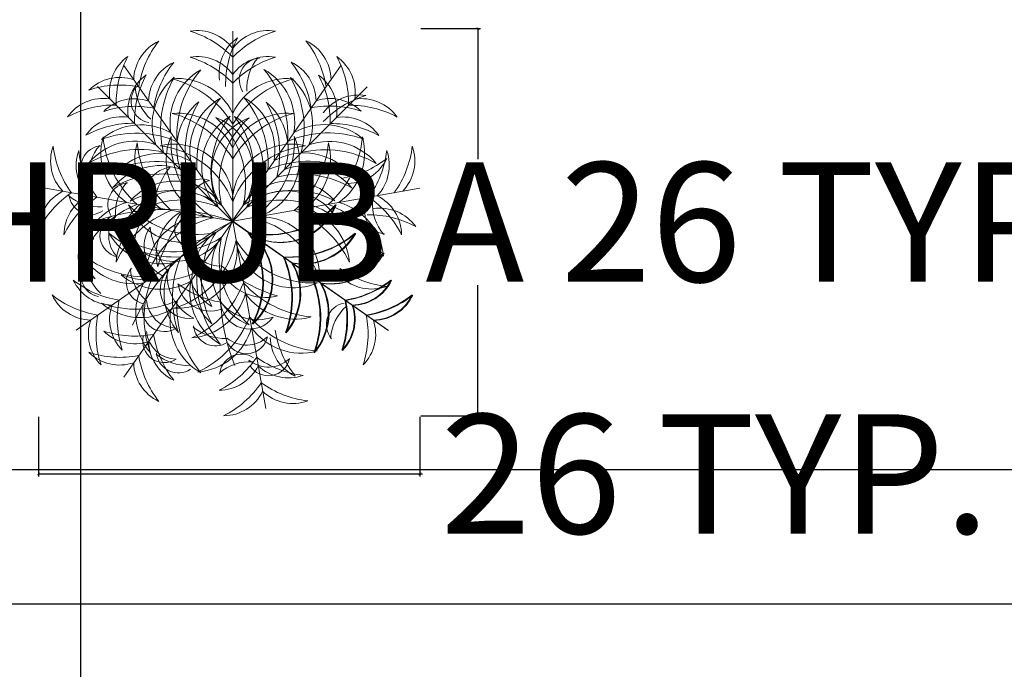
# Model space of a CAD drawing. Units: inches. Extents: x -48 to 50072, y 0 to 21068.
# Tile 5 of 75: x 212 to 278, y 210 to 253. Entities that reach past the tile are written whole.
import ezdxf

# ---------------------------------------------------------------- set-up
doc = ezdxf.new("R2010")
doc.units = ezdxf.units.IN
doc.header["$MEASUREMENT"] = 0
for name, color, linetype, lineweight in [('A-ANNO-DIMS', 2, 'Continuous', 18), ('C-PROP', 7, 'Continuous', 25), ('L-PLNT', 94, 'Continuous', 13)]:
    doc.layers.add(name, color=color, linetype=linetype, lineweight=lineweight)
doc.styles.get("Standard").update_dxf_attribs({"font": 'arial.ttf'})
doc.dimstyles.get("Standard").update_dxf_attribs({"dimtxt": 8, "dimasz": 0.18, "dimexe": 0.18, "dimexo": 0.0625, "dimgap": 0.09, "dimtad": 0, "dimtih": 1, "dimtoh": 1, "dimdec": 1, "dimzin": 0, "dimdsep": 46, "dimlunit": 4, "dimtxsty": 'Standard', "dimblk": 'ARCHTICK', "dimcen": 0.09, "dimadec": 0, "dimazin": 0, "dimtfac": 1, "dimtdec": 1, "dimtofl": 0, "dimtmove": 0, "dimatfit": 3, "dimldrblk": 'ARCHTICK', "dimfxl": 1, "dimtolj": 1, "dimtzin": 0, "dimarcsym": 0})

# ---------------------------------------------------------------- blocks, each defined once
blk = doc.blocks.new('A$C5D061C3B')
for p, q in [((3.377, 6.679), (3.377, 3.377)), ((1.483, 6.082), (3.377, 3.377)), ((5.259, 6.086), (3.365, 3.381)), ((1.03, 5.716), (3.365, 3.381)), ((5.712, 5.712), (3.377, 3.377)), ((0.125, 3.951), (3.377, 3.377)), ((6.629, 3.951), (3.377, 3.377)), ((0.66, 1.487), (3.365, 3.381)), ((1.483, 0.672), (3.377, 3.377)), ((6.07, 1.487), (3.365, 3.381)), ((3.951, 0.125), (3.377, 3.377)), ((6.082, 1.483), (3.377, 3.377))]:
    blk.add_line(p, q)
for centre, radius, start, end in [((2.763, 5.924), 0.762, 36.29, 99.6243), ((2.145, 5.032), 1.715, 44.0763, 73.3794), ((3.991, 5.924), 0.762, 80.3757, 143.71), ((4.61, 5.032), 1.715, 106.6206, 135.9237), ((2.419, 5.816), 0.762, 115.3757, 178.71), ((3.438, 5.44), 1.715, 141.6206, 170.9237), ((3.901, 5.939), 0.762, 125.3757, 188.71), ((4.969, 5.745), 1.715, 151.6206, 180.9237), ((3.305, 5.444), 1.715, 9.0763, 38.3794), ((4.323, 5.82), 0.762, 1.29, 64.6243), ((1.998, 5.617), 0.762, 125.3757, 188.71), ((3.066, 5.423), 1.715, 151.6206, 180.9237), ((2.763, 5.474), 0.762, 36.29, 99.6243), ((2.145, 4.581), 1.715, 44.0763, 73.3794), ((3.991, 5.474), 0.762, 80.3757, 143.71), ((4.61, 4.581), 1.715, 106.6206, 135.9237), ((3.871, 5.832), 0.38, 94.742, 213.7475), ((4.447, 5.681), 0.826, 139.618, 183.2106), ((4.744, 5.613), 0.762, 351.29, 54.6243), ((3.676, 5.419), 1.715, 359.0763, 28.3794), ((2.678, 5.447), 0.762, 115.3757, 178.71), ((3.696, 5.07), 1.715, 141.6206, 170.9237), ((3.344, 5.089), 1.056, 119.6063, 189.7511), ((4.177, 4.869), 1.77, 139.9634, 183.6288), ((3.398, 5.094), 1.056, 350.2489, 60.3937), ((2.565, 4.873), 1.77, 356.3712, 40.0366), ((4.064, 5.451), 0.762, 1.29, 64.6243), ((3.046, 5.075), 1.715, 9.0763, 38.3794), ((1.413, 5.111), 0.762, 71.29, 134.6243), ((2.317, 5.298), 0.762, 125.3757, 188.71), ((3.385, 5.104), 1.715, 151.6206, 180.9237), ((3.035, 5.062), 1.056, 129.6063, 199.7511), ((3.894, 4.989), 1.77, 149.9634, 193.6288), ((2.422, 4.799), 1.056, 25.2489, 95.3937), ((1.866, 4.14), 1.77, 31.3712, 75.0366), ((4.332, 4.799), 1.056, 84.6063, 154.7511), ((4.888, 4.14), 1.77, 104.9634, 148.6288), ((2.848, 4.985), 1.77, 346.3712, 30.0366), ((3.707, 5.058), 1.056, 340.2489, 50.3937), ((3.357, 5.1), 1.715, 359.0763, 28.3794), ((4.425, 5.294), 0.762, 351.29, 54.6243), ((1.419, 4.026), 1.715, 79.0763, 108.3794), ((1.991, 5.462), 0.38, 139.742, 258.7475), ((2.505, 5.763), 0.826, 184.618, 228.2106), ((1.13, 4.748), 0.762, 81.29, 144.6243), ((1.671, 4.742), 0.762, 71.29, 134.6243), ((3.688, 4.597), 1.056, 119.6063, 189.7511), ((4.522, 4.377), 1.77, 139.9634, 183.6288), ((2.221, 4.381), 1.77, 356.3712, 40.0366), ((3.054, 4.602), 1.056, 350.2489, 60.3937), ((5.071, 4.746), 0.762, 45.3757, 108.71), ((5.564, 4.807), 0.762, 80.3757, 143.71), ((6.182, 3.914), 1.715, 106.6206, 135.9237), ((5.613, 4.744), 0.762, 35.3757, 98.71), ((1.324, 3.68), 1.715, 89.0763, 118.3794), ((1.677, 3.657), 1.715, 79.0763, 108.3794), ((3.46, 4.637), 1.056, 129.6063, 199.7511), ((4.319, 4.565), 1.77, 149.9634, 193.6288), ((3.283, 4.633), 1.056, 340.2489, 50.3937), ((2.424, 4.56), 1.77, 346.3712, 30.0366), ((5.065, 3.661), 1.715, 71.6206, 100.9237), ((5.419, 3.676), 1.715, 61.6206, 90.9237), ((1.448, 4.43), 0.762, 81.29, 144.6243), ((2.422, 4.198), 1.056, 25.2489, 95.3937), ((1.866, 3.54), 1.77, 31.3712, 75.0366), ((3.868, 4.321), 1.029, 121.3654, 221.5741), ((4.556, 4.237), 1.557, 141.8122, 203.3335), ((4.035, 4.215), 1.029, 111.3654, 211.5741), ((2.707, 4.219), 1.029, 328.4259, 68.6346), ((2.044, 4.017), 1.557, 346.6665, 48.1878), ((4.698, 4.013), 1.557, 131.8122, 193.3335), ((4.332, 4.198), 1.056, 84.6063, 154.7511), ((4.888, 3.54), 1.77, 104.9634, 148.6288), ((2.187, 4.233), 1.557, 336.6665, 38.1878), ((2.875, 4.316), 1.029, 318.4259, 58.6346), ((5.294, 4.425), 0.762, 35.3757, 98.71), ((1.642, 3.362), 1.715, 89.0763, 118.3794), ((1.78, 3.994), 1.056, 60.2489, 130.3937), ((4.963, 3.998), 1.056, 49.6063, 119.7511), ((5.1, 3.357), 1.715, 61.6206, 90.9237), ((2.143, 4.564), 1.056, 164.6063, 234.7511), ((1.702, 3.136), 1.77, 66.3712, 110.0366), ((2.888, 4.998), 1.77, 184.9634, 228.6288), ((3.25, 4.435), 1.029, 156.3654, 256.5741), ((3.862, 4.761), 1.557, 176.8122, 238.3335), ((2.893, 4.761), 1.557, 301.6665, 3.1878), ((3.504, 4.435), 1.029, 283.4259, 23.6346), ((5.04, 3.14), 1.77, 69.9634, 113.6288), ((3.866, 4.998), 1.77, 311.3712, 355.0366), ((4.611, 4.564), 1.056, 305.2489, 15.3937), ((0.975, 4.424), 0.762, 160.3757, 223.71), ((1.962, 4.878), 1.715, 186.6206, 215.9237), ((1.12, 4.31), 0.38, 94.742, 213.7475), ((1.696, 4.159), 0.826, 139.618, 183.2106), ((1.685, 3.712), 1.056, 70.2489, 140.3937), ((1.757, 2.853), 1.77, 76.3712, 120.0366), ((2.734, 4.46), 1.056, 164.6063, 234.7511), ((3.48, 4.893), 1.77, 184.9634, 228.6288), ((2.358, 3.686), 1.029, 3.4259, 103.6346), ((1.93, 3.14), 1.557, 21.6665, 83.1878), ((4.397, 3.686), 1.029, 76.3654, 176.5741), ((4.824, 3.14), 1.557, 96.8122, 158.3335), ((3.275, 4.893), 1.77, 311.3712, 355.0366), ((4.02, 4.46), 1.056, 305.2489, 15.3937), ((5.058, 3.707), 1.056, 39.6063, 109.7511), ((4.793, 4.878), 1.715, 324.0763, 353.3794), ((5.779, 4.424), 0.762, 316.29, 19.6243), ((1.419, 4.346), 0.762, 160.3757, 223.71), ((2.405, 4.8), 1.715, 186.6206, 215.9237), ((2.124, 3.502), 1.056, 60.2489, 130.3937), ((4.618, 3.506), 1.056, 49.6063, 119.7511), ((4.985, 2.848), 1.77, 59.9634, 103.6288), ((4.988, 5.812), 1.715, 279.0763, 308.3794), ((5.365, 4.794), 0.762, 271.29, 334.6243), ((4.349, 4.8), 1.715, 324.0763, 353.3794), ((5.335, 4.346), 0.762, 316.29, 19.6243), ((2.109, 3.287), 1.056, 70.2489, 140.3937), ((2.046, 2.644), 1.77, 66.3712, 110.0366), ((2.387, 3.752), 0.574, 99.9865, 199.4034), ((3.599, 3.314), 1.651, 142.5759, 170.8942), ((4.696, 2.648), 1.77, 69.9634, 113.6288), ((4.633, 3.283), 1.056, 39.6063, 109.7511), ((2.182, 2.428), 1.77, 76.3712, 120.0366), ((2.84, 3.739), 0.372, 69.2257, 210.1279), ((4.56, 2.424), 1.77, 59.9634, 103.6288), ((1.588, 3.666), 0.38, 94.742, 213.7475), ((2.165, 3.515), 0.826, 139.618, 183.2106), ((2.365, 3.045), 1.029, 38.4259, 138.6346), ((3.109, 3.59), 0.515, 105.4398, 183.6694), ((4.377, 3.05), 1.029, 41.3654, 141.5741), ((0.762, 3.214), 0.762, 116.29, 179.6243), ((1.534, 2.451), 1.715, 124.0763, 153.3794), ((1.206, 3.136), 0.762, 116.29, 179.6243), ((1.977, 2.373), 1.715, 124.0763, 153.3794), ((1.062, 4.452), 0.826, 229.618, 273.2106), ((0.91, 3.875), 0.38, 184.742, 303.7475), ((2.426, 2.879), 1.029, 48.4259, 148.6346), ((2.328, 2.353), 1.557, 56.6665, 118.1878), ((4.414, 2.358), 1.557, 61.8122, 123.3335), ((4.316, 2.875), 1.029, 31.3654, 131.5741), ((4.777, 2.373), 1.715, 26.6206, 55.9237), ((5.549, 3.136), 0.762, 0.3757, 63.71), ((1.811, 2.684), 1.056, 105.2489, 175.3937), ((2.363, 2.022), 1.77, 111.3712, 155.0366), ((2.403, 2.58), 1.056, 105.2489, 175.3937), ((2.51, 2.191), 1.557, 66.6665, 128.1878), ((2.729, 4.702), 1.557, 221.8122, 283.3335), ((2.527, 4.039), 1.029, 201.3654, 301.5741), ((2.741, 3.253), 0.372, 114.2257, 255.1279), ((3.037, 3.338), 0.515, 150.4398, 228.6694), ((4.233, 2.187), 1.557, 51.8122, 113.3335), ((4.001, 4.702), 1.557, 256.6665, 318.1878), ((4.013, 4.698), 1.557, 256.6665, 318.1878), ((4.203, 4.039), 1.029, 238.4259, 338.6346), ((4.215, 4.035), 1.029, 238.4259, 338.6346), ((4.352, 2.58), 1.056, 4.6063, 74.7511), ((4.391, 2.022), 1.77, 24.9634, 68.6288), ((4.943, 2.684), 1.056, 4.6063, 74.7511), ((6.053, 3.533), 0.38, 146.2525, 265.258), ((6.629, 3.684), 0.826, 176.7894, 220.382), ((5.935, 2.842), 0.762, 35.3757, 98.71), ((2.185, 0.015), 3.567, 70.4772, 111.6585), ((1.447, 3.129), 0.376, 122.0577, 257.8533), ((1.751, 3.126), 0.529, 140.1845, 223.654), ((2.955, 1.917), 1.77, 111.3712, 155.0366), ((2.007, 3.071), 0.506, 93.8744, 233.9763), ((2.489, 2.932), 0.825, 128.7536, 199.097), ((2.896, 2.427), 1.029, 83.4259, 183.6346), ((3.359, 1.911), 1.557, 101.6665, 163.1878), ((2.903, 2.8), 0.855, 116.4477, 194.3672), ((4.744, 1.779), 2.789, 140.4007, 163.139), ((3.395, 1.911), 1.557, 16.8122, 78.3335), ((3.858, 2.427), 1.029, 356.3654, 96.5741), ((3.799, 1.917), 1.77, 24.9634, 68.6288), ((5.741, 1.774), 1.715, 61.6206, 90.9237), ((4.912, 0.157), 3.567, 115.4772, 156.6585), ((2.412, 2.943), 0.574, 144.9865, 244.4034), ((3.578, 3.49), 1.651, 187.5759, 215.8942), ((6.727, 2.189), 3.567, 160.4772, 201.6585), ((1.37, 2.745), 0.529, 140.1845, 223.654), ((2.145, 3.693), 1.056, 209.6063, 279.7511), ((2.365, 4.526), 1.77, 229.9634, 273.6288), ((2.328, 4.401), 1.557, 241.8122, 303.3335), ((3.697, 2.369), 1.029, 128.4259, 228.6346), ((4.389, 2.332), 1.557, 146.6665, 208.1878), ((4.698, 2.741), 1.557, 166.6665, 228.1878), ((2.341, 2.332), 1.557, 331.8122, 33.3335), ((2.353, 2.328), 1.557, 331.8122, 33.3335), ((3.033, 2.369), 1.029, 311.3654, 51.5741), ((3.045, 2.365), 1.029, 311.3654, 51.5741), ((4.365, 4.526), 1.77, 266.3712, 310.0366), ((4.377, 4.522), 1.77, 266.3712, 310.0366), ((4.585, 3.693), 1.056, 260.2489, 330.3937), ((4.597, 3.688), 1.056, 260.2489, 330.3937), ((1.067, 2.749), 0.376, 122.0577, 257.8533), ((2.365, 3.709), 1.029, 221.3654, 321.5741), ((1.911, 3.359), 1.557, 286.8122, 348.3335), ((2.427, 2.896), 1.029, 266.3654, 6.5741), ((3.003, 2.844), 0.372, 159.2257, 300.1279), ((3.152, 3.113), 0.515, 195.4398, 273.6694), ((5.474, 3.214), 2.789, 185.4007, 208.139), ((4.035, 2.539), 1.029, 148.4259, 248.6346), ((4.435, 3.25), 1.029, 193.4259, 293.6346), ((4.761, 3.862), 1.557, 211.6665, 273.1878), ((1.873, 4.181), 1.77, 229.9634, 273.6288), ((1.653, 3.348), 1.056, 209.6063, 279.7511), ((4.099, 2.051), 1.77, 156.3712, 200.0366), ((3.45, 2.634), 0.855, 161.4477, 239.3672), ((2.632, 2.051), 1.77, 339.9634, 23.6288), ((2.644, 2.046), 1.77, 339.9634, 23.6288), ((4.857, 4.181), 1.77, 266.3712, 310.0366), ((4.869, 4.177), 1.77, 266.3712, 310.0366), ((5.077, 3.348), 1.056, 260.2489, 330.3937), ((5.089, 3.344), 1.056, 260.2489, 330.3937), ((1.122, 2.441), 0.38, 139.742, 258.7475), ((1.636, 2.741), 0.826, 184.618, 228.2106), ((3.24, 2.128), 1.056, 150.2489, 220.3937), ((4.963, 4.749), 2.789, 230.4007, 253.139), ((3.49, 2.128), 1.056, 319.6063, 29.7511), ((3.502, 2.124), 1.056, 319.6063, 29.7511), ((2.046, 4.111), 1.77, 249.9634, 293.6288), ((2.124, 3.252), 1.056, 229.6063, 299.7511), ((1.908, 2.317), 0.38, 139.742, 258.7475), ((2.422, 2.617), 0.826, 184.618, 228.2106), ((3.607, 1.706), 1.77, 156.3712, 200.0366), ((2.624, 2.192), 0.506, 138.8744, 278.9763), ((3.064, 2.435), 0.825, 173.7536, 244.097), ((4.522, 2.378), 1.77, 176.3712, 220.0366), ((3.942, 2.908), 0.855, 206.4477, 284.3672), ((3.124, 1.706), 1.77, 339.9634, 23.6288), ((3.136, 1.702), 1.77, 339.9634, 23.6288), ((6.244, 3.948), 1.715, 234.0763, 263.3794), ((5.79, 2.962), 0.762, 226.29, 289.6243), ((1.672, 3.7), 1.715, 231.6206, 260.9237), ((1.295, 2.682), 0.762, 205.3757, 268.71), ((2.748, 1.784), 1.056, 150.2489, 220.3937), ((3.428, 3.603), 1.651, 232.5759, 260.8942), ((2.99, 2.391), 0.574, 189.9865, 289.4034), ((3.688, 2.157), 1.056, 170.2489, 240.3937), ((1.917, 2.955), 1.77, 294.9634, 338.6288), ((4.893, 3.48), 1.77, 221.3712, 265.0366), ((3.982, 1.784), 1.056, 319.6063, 29.7511), ((3.994, 1.78), 1.056, 319.6063, 29.7511), ((5.058, 3.7), 1.715, 279.0763, 308.3794), ((5.07, 3.696), 1.715, 279.0763, 308.3794), ((5.435, 2.682), 0.762, 271.29, 334.6243), ((5.447, 2.678), 0.762, 271.29, 334.6243), ((0.926, 2.424), 0.762, 205.3757, 268.71), ((1.303, 3.442), 1.715, 231.6206, 260.9237), ((2.58, 2.403), 1.056, 274.6063, 344.7511), ((4.46, 2.734), 1.056, 215.2489, 285.3937), ((5.427, 3.442), 1.715, 279.0763, 308.3794), ((5.44, 3.438), 1.715, 279.0763, 308.3794), ((5.804, 2.424), 0.762, 271.29, 334.6243), ((5.816, 2.419), 0.762, 271.29, 334.6243), ((1.702, 3.619), 1.77, 249.9634, 293.6288), ((1.78, 2.76), 1.056, 229.6063, 299.7511), ((2, 1.676), 0.762, 161.29, 224.6243), ((3.086, 1.681), 1.715, 169.0763, 198.3794), ((2.188, 1.837), 0.376, 167.0577, 302.8533), ((2.405, 2.049), 0.529, 185.1845, 268.654), ((4.177, 1.886), 1.77, 176.3712, 220.0366), ((3.81, 2.493), 0.825, 218.7536, 289.097), ((3.671, 2.011), 0.506, 183.8744, 323.9763), ((5.385, 1.584), 0.38, 101.2525, 220.258), ((5.899, 1.283), 0.826, 131.7894, 175.382), ((3.645, 1.681), 1.715, 341.6206, 10.9237), ((4.73, 1.676), 0.762, 315.3757, 18.71), ((3.657, 1.677), 1.715, 341.6206, 10.9237), ((4.742, 1.671), 0.762, 315.3757, 18.71), ((2.717, 1.423), 1.715, 169.0763, 198.3794), ((3.344, 1.665), 1.056, 170.2489, 240.3937), ((2.022, 2.363), 1.77, 294.9634, 338.6288), ((4.998, 2.888), 1.77, 221.3712, 265.0366), ((4.014, 1.423), 1.715, 341.6206, 10.9237), ((1.631, 1.417), 0.762, 161.29, 224.6243), ((3.227, 2.169), 0.826, 229.618, 273.2106), ((3.076, 1.593), 0.38, 184.742, 303.7475), ((5.099, 1.417), 0.762, 315.3757, 18.71), ((1.671, 2.012), 0.762, 225.3757, 288.71), ((1.677, 3.098), 1.715, 251.6206, 280.9237), ((2.188, 1.299), 0.376, 167.0577, 302.8533), ((2.405, 1.511), 0.529, 185.1845, 268.654), ((3.696, 1.684), 1.715, 189.0763, 218.3794), ((2.684, 1.811), 1.056, 274.6063, 344.7511), ((3.616, 1.755), 0.529, 230.1845, 313.654), ((3.613, 1.452), 0.376, 212.0577, 347.8533), ((4.564, 2.143), 1.056, 215.2489, 285.3937), ((5.808, 1.754), 1.715, 189.0763, 218.3794), ((2.678, 1.307), 0.762, 181.29, 244.6243), ((4.79, 1.377), 0.762, 181.29, 244.6243), ((1.419, 2.729), 1.715, 251.6206, 280.9237), ((1.413, 1.643), 0.762, 225.3757, 288.71), ((3.438, 1.315), 1.715, 189.0763, 218.3794), ((2.583, 1.701), 0.826, 229.618, 273.2106), ((2.432, 1.124), 0.38, 184.742, 303.7475), ((3.528, 0.69), 0.38, 56.2525, 175.258), ((2.419, 0.938), 0.762, 181.29, 244.6243), ((2.373, 1.977), 1.715, 296.6206, 325.9237), ((3.136, 1.206), 0.762, 270.3757, 333.71), ((3.68, 0.113), 0.826, 86.7894, 130.382), ((3.997, 1.374), 0.529, 230.1845, 313.654), ((3.994, 1.071), 0.376, 212.0577, 347.8533), ((4.8, 2.405), 1.715, 234.0763, 263.3794), ((4.346, 1.419), 0.762, 226.29, 289.6243), ((2.451, 1.534), 1.715, 296.6206, 325.9237), ((4.878, 1.962), 1.715, 234.0763, 263.3794), ((3.214, 0.762), 0.762, 270.3757, 333.71), ((4.424, 0.975), 0.762, 226.29, 289.6243)]:
    blk.add_arc(centre, radius, start, end)
blk = doc.blocks.new('_ArchTick')
at = {"color": 0, "linetype": 'ByBlock', "const_width": 0.15}
blk.add_lwpolyline([(-0.5, -0.5), (0.5, 0.5)], dxfattribs=at)
blk = doc.blocks.new('*D52')
at = {"layer": 'A-ANNO-DIMS', "color": 0, "lineweight": -2, "transparency": 16777216}
for p, q in [((238.847, 252.654), (242.859, 252.654)), ((242.679, 252.654), (242.679, 243.897)), ((242.679, 226.686), (242.679, 235.444)), ((238.847, 226.686), (242.859, 226.686))]:
    blk.add_line(p, q, dxfattribs=at)
at = {"layer": 'Defpoints', "color": 0, "transparency": 16777216}
for p in [(238.784, 252.654), (242.679, 252.654), (238.784, 226.686)]:
    blk.add_point(p, dxfattribs=at)
at = {"layer": 'A-ANNO-DIMS', "color": 0, "lineweight": -2, "transparency": 16777216, "xscale": 0.18, "yscale": 0.18, "zscale": 0.18}
for p, rotation in [((242.679, 252.654), 90), ((242.679, 226.686), 270)]:
    blk.add_blockref('_ArchTick', p, dxfattribs=dict(at, rotation=rotation))
at = {"layer": 'A-ANNO-DIMS', "color": 0, "transparency": 16777216, "insert": (242.679, 239.67), "char_height": 8, "attachment_point": 5}
blk.add_mtext('\\A1;SHRUB A 26 TYP.', dxfattribs=at)
blk = doc.blocks.new('*D53')
at = {"layer": 'A-ANNO-DIMS', "color": 0, "lineweight": -2, "transparency": 16777216}
for p, q in [((213.182, 226.623), (213.182, 222.61)), ((238.784, 226.623), (238.784, 222.61)), ((213.182, 222.79), (238.784, 222.79)), ((238.784, 222.79), (238.964, 222.79))]:
    blk.add_line(p, q, dxfattribs=at)
at = {"layer": 'Defpoints', "color": 0, "transparency": 16777216}
for p in [(213.182, 226.686), (238.784, 226.686), (238.784, 222.79)]:
    blk.add_point(p, dxfattribs=at)
at = {"layer": 'A-ANNO-DIMS', "color": 0, "lineweight": -2, "transparency": 16777216, "xscale": 0.18, "yscale": 0.18, "zscale": 0.18, "rotation": 180}
blk.add_blockref('_ArchTick', (213.182, 222.79), dxfattribs=at)
at = {"layer": 'A-ANNO-DIMS', "color": 0, "lineweight": -2, "transparency": 16777216, "xscale": 0.18, "yscale": 0.18, "zscale": 0.18}
blk.add_blockref('_ArchTick', (238.784, 222.79), dxfattribs=at)
at = {"layer": 'A-ANNO-DIMS', "color": 0, "transparency": 16777216, "insert": (258.593, 222.79), "char_height": 8, "attachment_point": 5}
blk.add_mtext('\\A1;26 TYP.', dxfattribs=at)
blk = doc.blocks.new('*D116')
at = {"layer": 'A-ANNO-DIMS', "color": 0, "lineweight": -2, "transparency": 16777216}
for p, q in [((18.017, 677.712), (18.017, 165.945)), ((216.017, 677.712), (216.017, 165.945)), ((18.017, 166.125), (108.458, 166.125)), ((216.017, 166.125), (125.576, 166.125))]:
    blk.add_line(p, q, dxfattribs=at)
at = {"layer": 'Defpoints', "color": 0, "transparency": 16777216}
for p in [(18.017, 677.775), (216.017, 677.775), (216.017, 166.125)]:
    blk.add_point(p, dxfattribs=at)
at = {"layer": 'A-ANNO-DIMS', "color": 0, "lineweight": -2, "transparency": 16777216, "xscale": 0.18, "yscale": 0.18, "zscale": 0.18, "rotation": 180}
blk.add_blockref('_ArchTick', (18.017, 166.125), dxfattribs=at)
at = {"layer": 'A-ANNO-DIMS', "color": 0, "lineweight": -2, "transparency": 16777216, "xscale": 0.18, "yscale": 0.18, "zscale": 0.18}
blk.add_blockref('_ArchTick', (216.017, 166.125), dxfattribs=at)
at = {"layer": 'A-ANNO-DIMS', "color": 0, "transparency": 16777216, "insert": (117.017, 166.125), "char_height": 8, "attachment_point": 5}
blk.add_mtext('\\A1;198', dxfattribs=at)
blk = doc.blocks.new('*D117')
at = {"layer": 'A-ANNO-DIMS', "color": 0, "lineweight": -2, "transparency": 16777216}
for p, q in [((216.017, 488.712), (216.017, 165.945)), ((297.017, 488.712), (297.017, 165.945)), ((216.017, 166.125), (251.464, 166.125)), ((297.017, 166.125), (261.57, 166.125))]:
    blk.add_line(p, q, dxfattribs=at)
at = {"layer": 'Defpoints', "color": 0, "transparency": 16777216}
for p in [(216.017, 488.775), (297.017, 488.775), (297.017, 166.125)]:
    blk.add_point(p, dxfattribs=at)
at = {"layer": 'A-ANNO-DIMS', "color": 0, "lineweight": -2, "transparency": 16777216, "xscale": 0.18, "yscale": 0.18, "zscale": 0.18, "rotation": 180}
blk.add_blockref('_ArchTick', (216.017, 166.125), dxfattribs=at)
at = {"layer": 'A-ANNO-DIMS', "color": 0, "lineweight": -2, "transparency": 16777216, "xscale": 0.18, "yscale": 0.18, "zscale": 0.18}
blk.add_blockref('_ArchTick', (297.017, 166.125), dxfattribs=at)
at = {"layer": 'A-ANNO-DIMS', "color": 0, "transparency": 16777216, "insert": (256.517, 166.125), "char_height": 8, "attachment_point": 5}
blk.add_mtext('\\A1;81', dxfattribs=at)

msp = doc.modelspace()

# ---------------------------------------------------------------- linework, layer by layer
at = {"layer": 'C-PROP'}
for p, q in [((210.389, 223.075), (544.517, 223.075)), ((210.389, 214.075), (553.517, 214.075))]:
    msp.add_line(p, q, dxfattribs=at)

# ---------------------------------------------------------------- block references
at = {"layer": 'L-PLNT', "xscale": 3.862191520948588, "yscale": 3.862191520948588, "zscale": 3.862191520948588}
msp.add_blockref('A$C5D061C3B', (213.182, 226.686), dxfattribs=at)

# ---------------------------------------------------------------- dimensions: what is measured, and where the dimension line sits
at = {"layer": 'A-ANNO-DIMS'}
for base, p1, p2, picture, middle in [((216.017, 166.125), (18.017, 677.775), (216.017, 677.775), '*D116', (117.017, 166.125)), ((297.017, 166.125), (216.017, 488.775), (297.017, 488.775), '*D117', (256.517, 166.125))]:
    dim = msp.add_linear_dim(base=base, p1=p1, p2=p2, dimstyle='Standard', override={"dimdec": 0, "dimlfac": 1, "dimrnd": 0, "dimzin": 0, "dimdsep": 46, "dimlunit": 2}, dxfattribs=at)
    dim.commit()
    dim.dimension.update_dxf_attribs({"geometry": picture, "text_midpoint": middle})
dim = msp.add_linear_dim(base=(242.679, 252.654), p1=(238.784, 226.686), p2=(238.784, 252.654), angle=90, text='SHRUB A <> TYP.', dimstyle='Standard', override={"dimdec": 0, "dimlfac": 1, "dimrnd": 0, "dimzin": 0, "dimdsep": 46, "dimlunit": 2}, dxfattribs=at)
dim.commit()
dim.dimension.update_dxf_attribs({"geometry": '*D52', "text_midpoint": (242.679, 239.67)})
dim = msp.add_linear_dim(base=(238.784, 222.79), p1=(213.182, 226.686), p2=(238.784, 226.686), text='<> TYP.', dimstyle='Standard', override={"dimdec": 0, "dimlfac": 1, "dimrnd": 0, "dimzin": 0, "dimdsep": 46, "dimlunit": 2}, dxfattribs=at)
dim.commit()
dim.dimension.update_dxf_attribs({"geometry": '*D53', "text_midpoint": (258.593, 222.79)})

doc.saveas('drawing.dxf')
